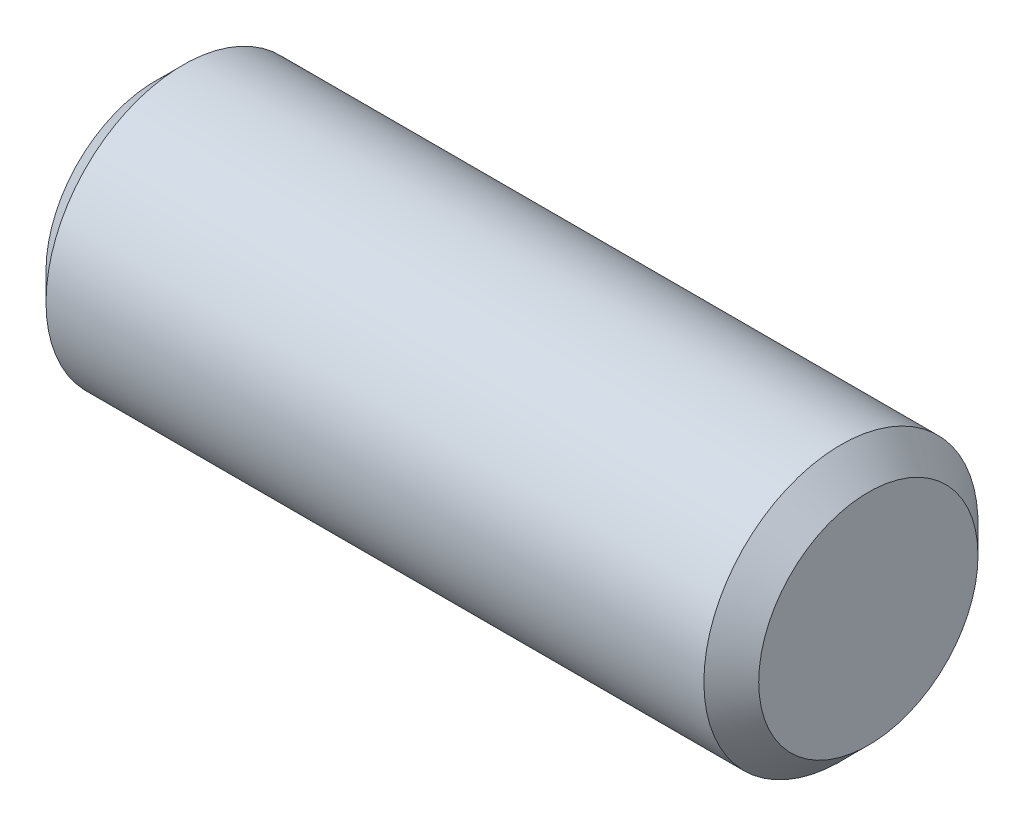
ISO-10303-21;
HEADER;
FILE_DESCRIPTION(('STEP AP214'),'2;1');
FILE_NAME('part.step','',(''),(''),'','','');
FILE_SCHEMA(('AUTOMOTIVE_DESIGN { 1 0 10303 214 1 1 1 1 }'));
ENDSEC;
DATA;
#1=APPLICATION_CONTEXT('core data for automotive mechanical design processes');
#2=APPLICATION_PROTOCOL_DEFINITION('international standard','automotive_design',2000,#1);
#3=PRODUCT_CONTEXT('',#1,'mechanical');
#4=PRODUCT('Part','Part','',(#3));
#5=PRODUCT_RELATED_PRODUCT_CATEGORY('part','',(#4));
#6=PRODUCT_DEFINITION_FORMATION('','',#4);
#7=PRODUCT_DEFINITION_CONTEXT('part definition',#1,'design');
#8=PRODUCT_DEFINITION('design','',#6,#7);
#9=PRODUCT_DEFINITION_SHAPE('','',#8);
#10=(LENGTH_UNIT() NAMED_UNIT(*) SI_UNIT(.MILLI.,.METRE.));
#11=(NAMED_UNIT(*) PLANE_ANGLE_UNIT() SI_UNIT($,.RADIAN.));
#12=(NAMED_UNIT(*) SI_UNIT($,.STERADIAN.) SOLID_ANGLE_UNIT());
#13=UNCERTAINTY_MEASURE_WITH_UNIT(LENGTH_MEASURE(1.E-05),#10,'distance_accuracy_value','');
#14=(GEOMETRIC_REPRESENTATION_CONTEXT(3) GLOBAL_UNCERTAINTY_ASSIGNED_CONTEXT((#13)) GLOBAL_UNIT_ASSIGNED_CONTEXT((#10,
#11,#12)) REPRESENTATION_CONTEXT('',''));
#15=CARTESIAN_POINT('',(0.,0.,0.));
#16=DIRECTION('',(0.,0.,1.));
#17=DIRECTION('',(1.,0.,0.));
#18=AXIS2_PLACEMENT_3D('',#15,#16,#17);
#19=CARTESIAN_POINT('',(26.,0.,0.));
#20=DIRECTION('',(-1.,0.,0.));
#21=DIRECTION('',(0.,0.,1.));
#22=AXIS2_PLACEMENT_3D('',#19,#20,#21);
#23=CYLINDRICAL_SURFACE('',#22,10.);
#24=CARTESIAN_POINT('',(-24.,0.,0.));
#25=DIRECTION('',(1.,0.,0.));
#26=DIRECTION('',(0.,0.,-1.));
#27=AXIS2_PLACEMENT_3D('',#24,#25,#26);
#28=CIRCLE('',#27,10.);
#29=CARTESIAN_POINT('',(-24.,0.,10.));
#30=VERTEX_POINT('',#29);
#31=EDGE_CURVE('E51',#30,#30,#28,.T.);
#32=CARTESIAN_POINT('',(24.,0.,0.));
#33=DIRECTION('',(1.,0.,0.));
#34=DIRECTION('',(0.,0.,-1.));
#35=AXIS2_PLACEMENT_3D('',#32,#33,#34);
#36=CIRCLE('',#35,10.);
#37=CARTESIAN_POINT('',(24.,0.,10.));
#38=VERTEX_POINT('',#37);
#39=EDGE_CURVE('E54',#38,#38,#36,.F.);
#40=CARTESIAN_POINT('',(-24.,0.,10.));
#41=CARTESIAN_POINT('',(-23.5,0.,10.));
#42=CARTESIAN_POINT('',(-23.,0.,10.));
#43=CARTESIAN_POINT('',(-22.,0.,10.));
#44=CARTESIAN_POINT('',(-21.5,0.,10.));
#45=CARTESIAN_POINT('',(-20.5,0.,10.));
#46=CARTESIAN_POINT('',(-20.,0.,10.));
#47=CARTESIAN_POINT('',(-19.,0.,10.));
#48=CARTESIAN_POINT('',(-18.5,0.,10.));
#49=CARTESIAN_POINT('',(-17.5,0.,10.));
#50=CARTESIAN_POINT('',(-17.,0.,10.));
#51=CARTESIAN_POINT('',(-16.,0.,10.));
#52=CARTESIAN_POINT('',(-15.5,0.,10.));
#53=CARTESIAN_POINT('',(-14.5,0.,10.));
#54=CARTESIAN_POINT('',(-14.,0.,10.));
#55=CARTESIAN_POINT('',(-13.,0.,10.));
#56=CARTESIAN_POINT('',(-12.5,0.,10.));
#57=CARTESIAN_POINT('',(-11.5,0.,10.));
#58=CARTESIAN_POINT('',(-11.,0.,10.));
#59=CARTESIAN_POINT('',(-9.99999999999996,0.,10.));
#60=CARTESIAN_POINT('',(-9.49999999999996,0.,10.));
#61=CARTESIAN_POINT('',(-8.49999999999996,0.,10.));
#62=CARTESIAN_POINT('',(-7.99999999999995,0.,10.));
#63=CARTESIAN_POINT('',(-6.99999999999995,0.,10.));
#64=CARTESIAN_POINT('',(-6.49999999999995,0.,10.));
#65=CARTESIAN_POINT('',(-5.49999999999995,0.,10.));
#66=CARTESIAN_POINT('',(-4.99999999999996,0.,10.));
#67=CARTESIAN_POINT('',(-3.99999999999996,0.,10.));
#68=CARTESIAN_POINT('',(-3.49999999999996,0.,10.));
#69=CARTESIAN_POINT('',(-2.49999999999996,0.,10.));
#70=CARTESIAN_POINT('',(-1.99999999999996,0.,10.));
#71=CARTESIAN_POINT('',(-0.999999999999959,0.,10.));
#72=CARTESIAN_POINT('',(-0.499999999999959,0.,10.));
#73=CARTESIAN_POINT('',(0.500000000000042,0.,10.));
#74=CARTESIAN_POINT('',(1.00000000000004,0.,10.));
#75=CARTESIAN_POINT('',(2.00000000000004,0.,10.));
#76=CARTESIAN_POINT('',(2.50000000000004,0.,10.));
#77=CARTESIAN_POINT('',(3.50000000000004,0.,10.));
#78=CARTESIAN_POINT('',(4.00000000000004,0.,10.));
#79=CARTESIAN_POINT('',(5.00000000000004,0.,10.));
#80=CARTESIAN_POINT('',(5.50000000000004,0.,10.));
#81=CARTESIAN_POINT('',(6.50000000000004,0.,10.));
#82=CARTESIAN_POINT('',(7.00000000000004,0.,10.));
#83=CARTESIAN_POINT('',(8.00000000000004,0.,10.));
#84=CARTESIAN_POINT('',(8.50000000000004,0.,10.));
#85=CARTESIAN_POINT('',(9.50000000000004,0.,10.));
#86=CARTESIAN_POINT('',(10.,0.,10.));
#87=CARTESIAN_POINT('',(11.,0.,10.));
#88=CARTESIAN_POINT('',(11.5,0.,10.));
#89=CARTESIAN_POINT('',(12.5,0.,10.));
#90=CARTESIAN_POINT('',(13.,0.,10.));
#91=CARTESIAN_POINT('',(14.,0.,10.));
#92=CARTESIAN_POINT('',(14.5,0.,10.));
#93=CARTESIAN_POINT('',(15.5,0.,10.));
#94=CARTESIAN_POINT('',(16.,0.,10.));
#95=CARTESIAN_POINT('',(17.,0.,10.));
#96=CARTESIAN_POINT('',(17.5,0.,10.));
#97=CARTESIAN_POINT('',(18.5,0.,10.));
#98=CARTESIAN_POINT('',(19.,0.,10.));
#99=CARTESIAN_POINT('',(20.,0.,10.));
#100=CARTESIAN_POINT('',(20.5,0.,10.));
#101=CARTESIAN_POINT('',(21.5,0.,10.));
#102=CARTESIAN_POINT('',(22.,0.,10.));
#103=CARTESIAN_POINT('',(23.,0.,10.));
#104=CARTESIAN_POINT('',(23.5,0.,10.));
#105=CARTESIAN_POINT('',(24.,0.,10.));
#106=B_SPLINE_CURVE_WITH_KNOTS('',3,(#40,#41,#42,#43,#44,#45,#46,#47,#48,#49,#50,#51,#52,#53,
#54,#55,#56,#57,#58,#59,#60,#61,#62,#63,#64,#65,#66,#67,#68,#69,#70,#71,#72,#73,#74,#75,#76,#77,
#78,#79,#80,#81,#82,#83,#84,#85,#86,#87,#88,#89,#90,#91,#92,#93,#94,#95,#96,#97,#98,#99,#100,
#101,#102,#103,#104,#105),.UNSPECIFIED.,.F.,.F.,(4,2,2,2,2,2,2,2,2,2,2,2,2,2,2,2,2,2,2,2,2,2,2,
2,2,2,2,2,2,2,2,2,4),(0.,1.5,3.,4.5,6.,7.5,9.,10.5,12.,13.5,15.,16.5,18.,19.5,21.,22.5,24.,25.5,
27.,28.5,30.,31.5,33.,34.5,36.,37.5,39.,40.5,42.,43.5,45.,46.5,48.),.UNSPECIFIED.);
#107=EDGE_CURVE('BSEAM39',#30,#38,#106,.T.);
#108=ORIENTED_EDGE('',*,*,#31,.T.);
#109=ORIENTED_EDGE('',*,*,#39,.T.);
#110=ORIENTED_EDGE('',*,*,#107,.T.);
#111=ORIENTED_EDGE('',*,*,#107,.F.);
#112=EDGE_LOOP('',(#108,#110,#109,#111));
#113=FACE_BOUND('',#112,.T.);
#114=ADVANCED_FACE('F39',(#113),#23,.T.);
#115=CARTESIAN_POINT('',(26.,0.,0.));
#116=DIRECTION('',(1.,0.,0.));
#117=DIRECTION('',(0.,0.,-1.));
#118=AXIS2_PLACEMENT_3D('',#115,#116,#117);
#119=PLANE('',#118);
#120=CARTESIAN_POINT('',(26.,0.,0.));
#121=DIRECTION('',(1.,0.,0.));
#122=DIRECTION('',(0.,0.,-1.));
#123=AXIS2_PLACEMENT_3D('',#120,#121,#122);
#124=CIRCLE('',#123,8.00000000000005);
#125=CARTESIAN_POINT('',(26.,0.,-8.00000000000005));
#126=VERTEX_POINT('',#125);
#127=EDGE_CURVE('E10',#126,#126,#124,.T.);
#128=ORIENTED_EDGE('',*,*,#127,.T.);
#129=EDGE_LOOP('',(#128));
#130=FACE_BOUND('',#129,.T.);
#131=ADVANCED_FACE('F72',(#130),#119,.T.);
#132=CARTESIAN_POINT('',(-26.,0.,0.));
#133=DIRECTION('',(1.,0.,0.));
#134=DIRECTION('',(0.,0.,-1.));
#135=AXIS2_PLACEMENT_3D('',#132,#133,#134);
#136=PLANE('',#135);
#137=CARTESIAN_POINT('',(-26.,0.,0.));
#138=DIRECTION('',(1.,0.,0.));
#139=DIRECTION('',(0.,0.,-1.));
#140=AXIS2_PLACEMENT_3D('',#137,#138,#139);
#141=CIRCLE('',#140,7.99999999999995);
#142=CARTESIAN_POINT('',(-26.,0.,-7.99999999999995));
#143=VERTEX_POINT('',#142);
#144=EDGE_CURVE('E50',#143,#143,#141,.F.);
#145=ORIENTED_EDGE('',*,*,#144,.T.);
#146=EDGE_LOOP('',(#145));
#147=FACE_BOUND('',#146,.T.);
#148=ADVANCED_FACE('F69',(#147),#136,.F.);
#149=CARTESIAN_POINT('',(-24.,0.,0.));
#150=DIRECTION('',(1.,0.,0.));
#151=DIRECTION('',(0.,0.,-1.));
#152=AXIS2_PLACEMENT_3D('',#149,#150,#151);
#153=CONICAL_SURFACE('',#152,10.,0.78539816339745);
#154=ORIENTED_EDGE('',*,*,#144,.F.);
#155=EDGE_LOOP('',(#154));
#156=FACE_BOUND('',#155,.T.);
#157=ORIENTED_EDGE('',*,*,#31,.F.);
#158=EDGE_LOOP('',(#157));
#159=FACE_BOUND('',#158,.T.);
#160=ADVANCED_FACE('F63',(#156,#159),#153,.T.);
#161=CARTESIAN_POINT('',(26.,0.,0.));
#162=DIRECTION('',(-1.,0.,0.));
#163=DIRECTION('',(0.,0.,1.));
#164=AXIS2_PLACEMENT_3D('',#161,#162,#163);
#165=CONICAL_SURFACE('',#164,8.00000000000005,0.785398163397447);
#166=ORIENTED_EDGE('',*,*,#39,.F.);
#167=EDGE_LOOP('',(#166));
#168=FACE_BOUND('',#167,.T.);
#169=ORIENTED_EDGE('',*,*,#127,.F.);
#170=EDGE_LOOP('',(#169));
#171=FACE_BOUND('',#170,.T.);
#172=ADVANCED_FACE('F45',(#168,#171),#165,.T.);
#173=CLOSED_SHELL('',(#114,#131,#148,#160,#172));
#174=MANIFOLD_SOLID_BREP('B2',#173);
#175=ADVANCED_BREP_SHAPE_REPRESENTATION('',(#18,#174),#14);
#176=SHAPE_DEFINITION_REPRESENTATION(#9,#175);
ENDSEC;
END-ISO-10303-21;
